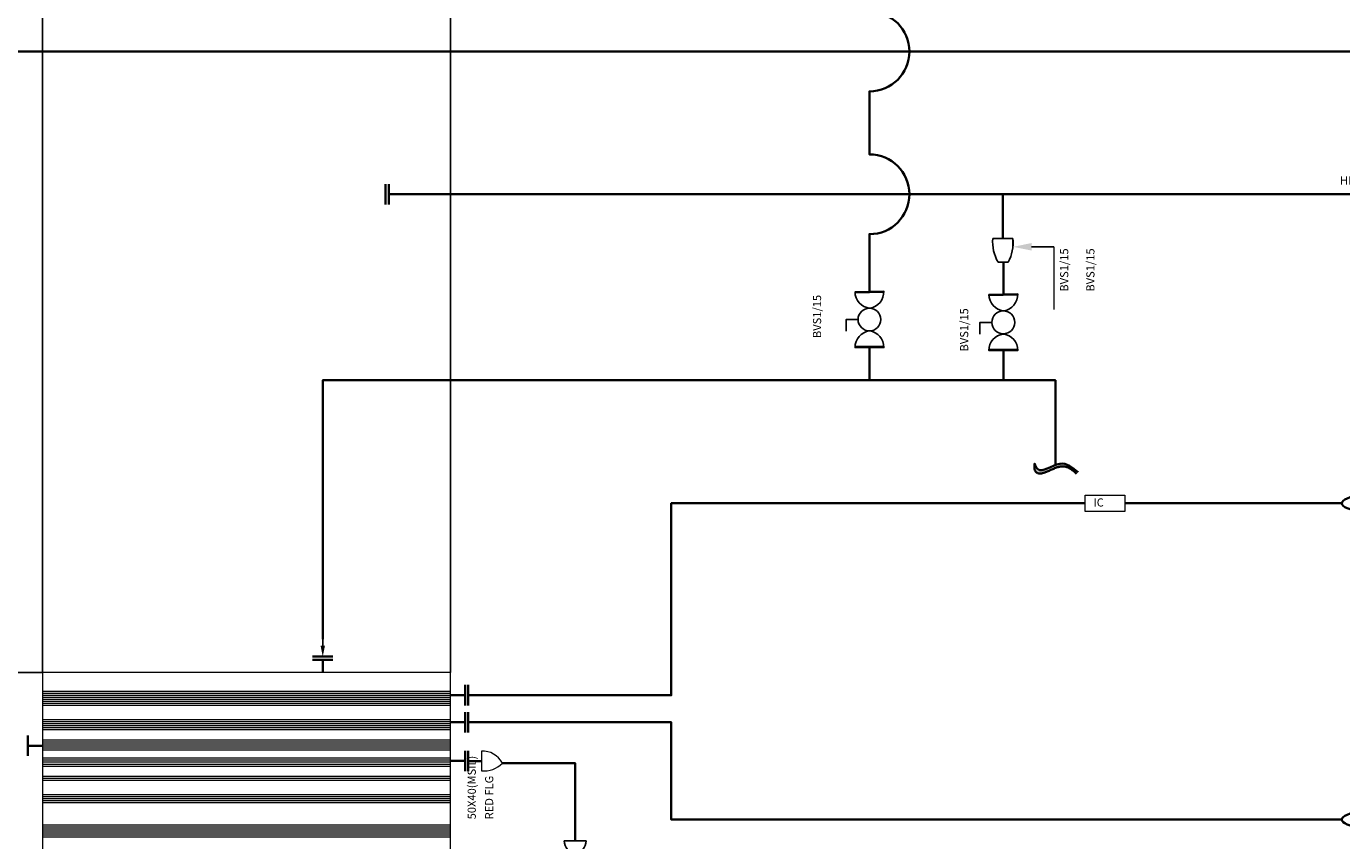
# Model space of a CAD drawing. Units: millimetres. Extents: x 353872 to 441597, y 126154 to 187356.
# Tile 24 of 28: x 399262 to 415084, y 165906 to 175703. Entities that reach past the tile are written whole.
import ezdxf

# ---------------------------------------------------------------- set-up
doc = ezdxf.new("R2010")
doc.units = ezdxf.units.MM
for name, color, linetype, lineweight in [('A-ANNO-DIMS', 2, 'Continuous', 18), ('P-ANNO-SYMB', 7, 'Continuous', 18), ('P-ANNO-TEXT', 7, 'Continuous', 25), ('P-INST-SIGN', 4, 'Continuous', 18), ('P-PIPE', 3, 'Continuous', 35), ('P-PIPE-FITT', 6, 'Continuous', 25), ('P-SYMB-PATT', 8, 'Continuous', 13), ('P-VALV', 2, 'Continuous', 25)]:
    doc.layers.add(name, color=color, linetype=linetype, lineweight=lineweight)
doc.layers.add('AC-UINT', color=2, linetype='Continuous')
doc.styles.get("Standard").update_dxf_attribs({"font": 'arial.ttf'})
doc.dimstyles.get("Standard").update_dxf_attribs({"dimtxt": 0.18, "dimasz": 0.18, "dimexe": 0.18, "dimexo": 0.0625, "dimgap": 0.09, "dimtad": 0, "dimtih": 1, "dimtoh": 1, "dimdec": 4, "dimzin": 0, "dimdsep": 46, "dimtxsty": 'Standard', "dimcen": 0.09, "dimadec": 0, "dimazin": 0, "dimtfac": 1, "dimtdec": 4, "dimtofl": 0, "dimtmove": 0, "dimatfit": 3, "dimfxl": 1, "dimtolj": 1, "dimtzin": 0, "dimarcsym": 0})

# ---------------------------------------------------------------- blocks, each defined once
blk = doc.blocks.new('DFSG')
at = {"layer": 'AC-UINT', "ltscale": 3}
blk.add_line((94.324, -27.16), (94.091, -27.16), dxfattribs=at)
blk.add_solid([(94.091, -27.121), (94.091, -27.199), (93.897, -27.16)], dxfattribs=at)
blk = doc.blocks.new('VALVE-B')
for points in [[(0, 12), (347, 12)], [(0, 8), (347, 8)], [(0, 4), (0, 0), (347, 0), (347, 5)], [(0, 4), (0, 4), (343, 4), (347, 4)]]:
    blk.add_lwpolyline(points)
for centre, radius, start, end in [((199, 2), 199, 97.3612, 180.5798), ((149, 3), 198, 359.2193, 82.8397)]:
    blk.add_arc(centre, radius, start, end)
blk = doc.blocks.new('VALVE-P')
blk.add_lwpolyline([(264, 173), (0, 173)])
for centre, radius, start, end in [((199, 188), 200, 184.2463, 250.3444), ((64, 189), 201, 289.8639, 355.5453)]:
    blk.add_arc(centre, radius, start, end)
blk = doc.blocks.new('*D33')
at = {"layer": 'A-ANNO-DIMS', "color": 0, "lineweight": -2, "transparency": 16777216}
for p, q in [((399457, 167930), (399457, 186546)), ((399457, 186546), (401910, 186546)), ((404363, 186546), (401911, 186546)), ((404363, 167930), (404363, 186546))]:
    blk.add_line(p, q, dxfattribs=at)
at = {"layer": 'A-ANNO-DIMS', "color": 0, "transparency": 16777216}
for points in [[(399457, 186546), (399457, 186546), (399457, 186546)], [(404363, 186546), (404363, 186546), (404363, 186546)]]:
    blk.add_solid(points, dxfattribs=at)
at = {"layer": 'Defpoints', "color": 0, "transparency": 16777216}
for p in [(404363, 186546), (399457, 167930), (404363, 167930)]:
    blk.add_point(p, dxfattribs=at)
at = {"layer": 'A-ANNO-DIMS', "color": 0, "transparency": 16777216, "insert": (401910, 186546), "char_height": 0.18, "attachment_point": 5}
blk.add_mtext('\\A1;4906', dxfattribs=at)
blk = doc.blocks.new('*D34')
at = {"layer": 'A-ANNO-DIMS', "color": 0, "lineweight": -2, "transparency": 16777216}
for p, q in [((399457, 167930), (356736, 167930)), ((356737, 167930), (356737, 163994)), ((356737, 160058), (356737, 163994)), ((399457, 160058), (356736, 160058))]:
    blk.add_line(p, q, dxfattribs=at)
at = {"layer": 'A-ANNO-DIMS', "color": 0, "transparency": 16777216}
for points in [[(356737, 167930), (356737, 167930), (356737, 167930)], [(356737, 160058), (356737, 160058), (356737, 160058)]]:
    blk.add_solid(points, dxfattribs=at)
at = {"layer": 'Defpoints', "color": 0, "transparency": 16777216}
for p in [(399457, 167930), (356737, 160058), (399457, 160058)]:
    blk.add_point(p, dxfattribs=at)
at = {"layer": 'A-ANNO-DIMS', "color": 0, "transparency": 16777216, "insert": (356737, 163994), "char_height": 0.18, "attachment_point": 5}
blk.add_mtext('\\A1;7872', dxfattribs=at)

msp = doc.modelspace()

# ---------------------------------------------------------------- hatches: boundary and pattern name
at = {"layer": 'P-SYMB-PATT'}
h = msp.add_hatch(color=256, dxfattribs=at)
h.dxf.hatch_style = 1
edge = h.paths.add_edge_path()
edge.add_spline(control_points=[(411390.89, 170443.52), (411390.67, 170440.97), (411390.44, 170438.39), (411389.76, 170430.59), (411389.33, 170425.32), (411388.62, 170414.26), (411388.36, 170408.48), (411388.27, 170396.91), (411388.44, 170391.13), (411389.36, 170382.04), (411389.81, 170378.82), (411390.94, 170373.15), (411391.51, 170370.72), (411392.96, 170365.81), (411393.81, 170363.36), (411396.48, 170356.98), (411398.56, 170353.08), (411403.61, 170345.73), (411406.6, 170342.29), (411413.25, 170336.23), (411416.92, 170333.63), (411424.5, 170329.4), (411428.41, 170327.76), (411436.16, 170325.33), (411440, 170324.52), (411447.5, 170323.5), (411451.17, 170323.28), (411461.46, 170323.25), (411467.9, 170323.94), (411480.65, 170326.14), (411486.96, 170327.66), (411499.68, 170331.29), (411506.08, 170333.4), (411519.07, 170338.07), (411525.65, 170340.62), (411546.51, 170349.09), (411561.13, 170355.56), (411590.78, 170368.69), (411605.81, 170375.36), (411635.44, 170387.63), (411650.05, 170393.24), (411670.51, 170399.85), (411676.94, 170401.73), (411687.59, 170404.43), (411691.93, 170405.39), (411699.54, 170406.83), (411702.88, 170407.37), (411709.47, 170408.22), (411712.7, 170408.53), (411722.23, 170409.19), (411728.37, 170409.22), (411744.84, 170408.35), (411754.86, 170406.72), (411774.52, 170401.58), (411784.16, 170398.07), (411803.36, 170389.36), (411812.91, 170384.17), (411832.06, 170372.4), (411841.65, 170365.83), (411864.69, 170349.03), (411878.19, 170338.36), (411893.02, 170320.82)], knot_values=[0, 0, 0, 0, 1.45657696, 1.45657696, 4.36973087, 4.36973087, 7.5343006, 7.5343006, 10.69887033, 10.69887033, 12.40671205, 12.40671205, 13.63901259, 13.63901259, 14.87131314, 14.87131314, 16.90061252, 16.90061252, 18.92991189, 18.92991189, 20.95921127, 20.95921127, 22.98851065, 22.98851065, 25.01781003, 25.01781003, 27.04710941, 27.04710941, 30.82532254, 30.82532254, 34.60353567, 34.60353567, 38.38174881, 38.38174881, 42.15996194, 42.15996194, 50.18983557, 50.18983557, 58.21970919, 58.21970919, 66.24958282, 66.24958282, 70.07411996, 70.07411996, 72.8401263, 72.8401263, 75.12034604, 75.12034604, 77.40056578, 77.40056578, 81.96100526, 81.96100526, 89.95516575, 89.95516575, 97.94932623, 97.94932623, 105.94348671, 105.94348671, 113.9376472, 113.9376472, 125.00201057, 125.00201057, 125.00201057, 125.00201057], degree=3, periodic=0)
edge.add_line((411893.02, 170320.82), (411913.35, 170339.3))
edge.add_spline(control_points=[(411913.35, 170339.3), (411845.38, 170395.98), (411763.83, 170463.97), (411657.92, 170432.84), (411640.09, 170426.25)], knot_values=[65.29657048, 65.29657048, 65.29657048, 65.29657048, 118.21354525, 128.78520648, 128.78520648, 128.78520648, 128.78520648], degree=3, periodic=0)
edge.add_spline(control_points=[(411640.09, 170426.25), (411557, 170395.56), (411440.95, 170314.41), (411400.77, 170418.04), (411390.89, 170443.52)], knot_values=[0, 0, 0, 0, 49.23816608, 65.29657048, 65.29657048, 65.29657048, 65.29657048], degree=3, periodic=0)

# ---------------------------------------------------------------- linework, layer by layer
at = {"layer": 'P-ANNO-SYMB'}
msp.add_line((411623.42, 173050.35), (411623.42, 172295.58), dxfattribs=at)
at = {"layer": 'P-INST-SIGN'}
for p, q in [((399457.15, 167706.61), (404363.17, 167706.61)), ((399457.15, 167682.23), (404363.17, 167682.23)), ((399457.15, 167657.84), (404363.17, 167657.84)), ((399457.15, 167633.45), (404363.17, 167633.45)), ((399457.15, 167633.45), (404363.17, 167633.45)), ((399457.15, 167609.06), (404363.17, 167609.06)), ((399457.15, 167584.67), (404363.17, 167584.67)), ((399457.15, 167560.28), (404363.17, 167560.28)), ((399457.15, 167560.28), (404363.17, 167560.28)), ((399457.15, 167535.9), (404363.17, 167535.9)), ((399457.15, 167365.18), (404363.17, 167365.18)), ((399457.15, 167340.79), (404363.17, 167340.79)), ((399457.15, 167316.4), (404363.17, 167316.4)), ((399457.15, 167292.01), (404363.17, 167292.01)), ((399457.15, 167267.62), (404363.17, 167267.62)), ((399457.15, 167243.23), (404363.17, 167243.23)), ((399457.15, 167121.29), (404363.17, 167121.29)), ((399457.15, 167096.9), (404363.17, 167096.9)), ((399457.15, 167072.52), (404363.17, 167072.52)), ((399457.15, 167048.13), (404363.17, 167048.13)), ((399457.15, 167023.74), (404363.17, 167023.74)), ((399457.15, 166999.35), (404363.17, 166999.35)), ((404736.17, 166983.02), (404736.17, 166745.9)), ((399457.15, 166901.8), (404363.17, 166901.8)), ((399457.15, 166877.41), (404363.17, 166877.41)), ((399457.15, 166853.02), (404363.17, 166853.02)), ((399457.15, 166828.63), (404363.17, 166828.63)), ((399457.15, 166804.24), (404363.17, 166804.24)), ((399457.15, 166682.3), (404363.17, 166682.3)), ((399457.15, 166657.91), (404363.17, 166657.91)), ((399457.15, 166657.91), (404363.17, 166657.91)), ((399457.15, 166633.52), (404363.17, 166633.52)), ((399457.15, 166462.8), (404363.17, 166462.8)), ((399457.15, 166438.42), (404363.17, 166438.42)), ((399457.15, 166414.03), (404363.17, 166414.03)), ((399457.15, 166389.64), (404363.17, 166389.64)), ((399457.15, 166365.25), (404363.17, 166365.25)), ((399457.15, 166096.98), (404363.17, 166096.98)), ((399457.15, 166072.59), (404363.17, 166072.59)), ((399457.15, 166048.2), (404363.17, 166048.2)), ((399457.15, 166048.2), (404363.17, 166048.2)), ((399457.15, 166023.81), (404363.17, 166023.81)), ((399457.15, 165999.42), (404363.17, 165999.42)), ((399457.15, 165975.04), (404363.17, 165975.04)), ((399457.15, 165950.65), (404363.17, 165950.65))]:
    msp.add_line(p, q, dxfattribs=at)
for points in [[(411999.14, 170063.27), (412475.78, 170063.27), (412475.78, 169866.13), (411999.14, 169866.13)], [(404363.17, 167929.97), (399457.15, 167929.97), (399457.15, 160058.19), (404363.17, 160058.19)]]:
    msp.add_lwpolyline(points, close=True, dxfattribs=at)
for centre, radius, start, end in [((404752.45, 166718.18), 265.34, 27.376995, 93.518711), ((404764.38, 167054.18), 309.56, 264.770963, 316.27178)]:
    msp.add_arc(centre, radius, start, end, dxfattribs=at)
at = {"layer": 'P-PIPE'}
for p, q in [((403583.29, 173805.12), (403583.29, 173560.36)), ((403622.45, 173805.12), (403622.45, 173560.36)), ((426420.76, 173682.74), (403622.45, 173682.74)), ((411008.36, 173150.27), (411008.36, 173682.74)), ((411014.55, 172476.18), (411014.55, 172864.89)), ((409404.23, 171839.16), (409404.23, 171444.56)), ((411014.53, 171789.73), (411014.53, 171444.56)), ((415084.48, 169964.7), (412475.78, 169964.7)), ((402950.3, 168120.52), (402705.54, 168120.52)), ((402950.3, 168081.36), (402705.54, 168081.36)), ((402827.92, 168081.36), (402827.92, 167929.97)), ((404538.96, 167779.19), (404538.96, 167534.43)), ((404578.12, 167779.19), (404578.12, 167534.43)), ((404363.17, 167657.84), (404538.96, 167657.84)), ((404538.96, 167452.85), (404538.96, 167208.09)), ((404578.12, 167452.85), (404578.12, 167208.09)), ((404363.17, 167331.49), (404538.96, 167331.49)), ((399281.36, 166926.77), (399281.36, 167171.53)), ((399457.15, 167048.13), (399281.36, 167048.13)), ((404538.96, 166986.76), (404538.96, 166742)), ((404578.12, 166986.76), (404578.12, 166742)), ((404363.17, 166865.41), (404538.96, 166865.41)), ((404578.12, 166864.38), (404736.17, 166864.38))]:
    msp.add_line(p, q, dxfattribs=at)
msp.add_lwpolyline([(426420.76, 177114.41), (409404.23, 177114.41), (409404.23, 175879.94, -1), (409404.23, 174919.83), (409404.23, 174162.79, -1), (409404.23, 173202.69), (409404.23, 172914.66), (409404.23, 172512.05)], format="xyb", dxfattribs=at)
for points in [[(393066.71, 149319.73), (393066.71, 175399.89), (426420.76, 175399.89)], [(402828.13, 168331.12), (402827.92, 171444.56), (411640.09, 171444.56), (411640.09, 170426.25)], [(411999.14, 169964.7), (407132.63, 169964.7), (407019.22, 169964.7), (407019.22, 167656.81), (405749.06, 167656.81), (404578.12, 167656.81)], [(415084.48, 166160.17), (411014.25, 166160.17), (407019.22, 166160.17), (407019.22, 167330.47), (404578.12, 167330.47)], [(404988.08, 166840.2), (405863.95, 166840.2), (405863.95, 165906.19)]]:
    msp.add_lwpolyline(points, dxfattribs=at)
for centre in [(415913.9, 169964.7), (415913.9, 169964.7), (415913.9, 166160.17), (415913.9, 166160.17)]:
    msp.add_ellipse(centre, major_axis=(829.42, 0), ratio=0.18269243, dxfattribs=at)
msp.add_open_spline([(411913.35, 170339.3), (411845.38, 170395.98), (411700.58, 170516.7), (411447.45, 170297.63), (411400.77, 170418.04), (411390.89, 170443.52), (411390.67, 170440.97), (411390.44, 170438.39), (411389.76, 170430.59), (411389.33, 170425.32), (411388.62, 170414.26), (411388.36, 170408.48), (411388.27, 170396.91), (411388.44, 170391.13), (411389.36, 170382.04), (411389.81, 170378.82), (411390.94, 170373.15), (411391.51, 170370.72), (411392.96, 170365.81), (411393.81, 170363.36), (411396.48, 170356.98), (411398.56, 170353.08), (411403.61, 170345.73), (411406.6, 170342.29), (411413.25, 170336.23), (411416.92, 170333.63), (411424.5, 170329.4), (411428.41, 170327.76), (411436.16, 170325.33), (411440, 170324.52), (411447.5, 170323.5), (411451.17, 170323.28), (411461.46, 170323.25), (411467.9, 170323.94), (411480.65, 170326.14), (411486.96, 170327.66), (411499.68, 170331.29), (411506.08, 170333.4), (411519.07, 170338.07), (411525.65, 170340.62), (411546.51, 170349.09), (411561.13, 170355.56), (411590.78, 170368.69), (411605.81, 170375.36), (411635.44, 170387.63), (411650.05, 170393.24), (411670.51, 170399.85), (411676.94, 170401.73), (411687.59, 170404.43), (411691.93, 170405.39), (411699.54, 170406.83), (411702.88, 170407.37), (411709.47, 170408.22), (411712.7, 170408.53), (411722.23, 170409.19), (411728.37, 170409.22), (411744.84, 170408.35), (411754.86, 170406.72), (411774.52, 170401.58), (411784.16, 170398.07), (411803.36, 170389.36), (411812.91, 170384.17), (411832.06, 170372.4), (411841.65, 170365.83), (411864.69, 170349.03), (411878.19, 170338.36), (411893.02, 170320.82)], degree=3, knots=[0, 0, 0, 0, 346.87515529, 738.93353045, 844.19770217, 844.19770217, 844.19770217, 845.65427913, 845.65427913, 848.56743304, 848.56743304, 851.73200277, 851.73200277, 854.8965725, 854.8965725, 856.60441422, 856.60441422, 857.83671477, 857.83671477, 859.06901531, 859.06901531, 861.09831469, 861.09831469, 863.12761407, 863.12761407, 865.15691345, 865.15691345, 867.18621283, 867.18621283, 869.2155122, 869.2155122, 871.24481158, 871.24481158, 875.02302472, 875.02302472, 878.80123785, 878.80123785, 882.57945098, 882.57945098, 886.35766411, 886.35766411, 894.38753774, 894.38753774, 902.41741137, 902.41741137, 910.44728499, 910.44728499, 914.27182214, 914.27182214, 917.03782847, 917.03782847, 919.31804821, 919.31804821, 921.59826795, 921.59826795, 926.15870744, 926.15870744, 934.15286792, 934.15286792, 942.1470284, 942.1470284, 950.14118889, 950.14118889, 958.13534937, 958.13534937, 969.19971274, 969.19971274, 969.19971274, 969.19971274], dxfattribs=at)
at = {"layer": 'P-VALV'}
for p, q in [((411130.35, 173150.27), (410886.38, 173150.27)), ((411130.35, 173058.5), (411130.35, 173151.98))]:
    msp.add_line(p, q, dxfattribs=at)
for points in [[(410950.47, 172864.89), (411014.55, 172864.89), (411072.45, 172864.89)], [(409266.91, 172175.6), (409123.61, 172175.6), (409123.61, 172034.91)], [(410876.15, 172141), (410731.72, 172141), (410731.72, 171999.19)]]:
    msp.add_lwpolyline(points, dxfattribs=at)
for centre, radius in [((409403.76, 172175.6), 136.85), ((411014.08, 172141), 137.93)]:
    msp.add_circle(centre, radius, dxfattribs=at)
for centre, radius, start, end in [((411379.15, 173111.03), 494.32, 175.447638, 209.864188), ((410628.49, 173103.52), 504.03, 331.741199, 5.321321)]:
    msp.add_arc(centre, radius, start, end, dxfattribs=at)

# ---------------------------------------------------------------- block references
at = {"layer": 'P-PIPE-FITT', "xscale": 1154.295526641529, "yscale": 1154.295526641529, "zscale": 1154.295526641529}
msp.add_blockref('DFSG', (302746.01, 204401.14), dxfattribs=at)
at = {"layer": 'P-PIPE-FITT', "xscale": 677.5688707767378, "yscale": 677.5688707767378, "zscale": 677.5688707767378, "rotation": 90.000000000006}
msp.add_blockref('DFSG', (384425.28, 104499.16), dxfattribs=at)
at = {"layer": 'P-VALV'}
for p, rotation in [((409577.1, 172515.99), 181.3019170021721), ((411187.42, 172483.84), 181.301917002174)]:
    msp.add_blockref('VALVE-B', p, dxfattribs=dict(at, rotation=rotation))
for name, p in [('VALVE-B', (409230.59, 171839.16)), ('VALVE-B', (410840.92, 171802.1)), ('VALVE-P', (405732.05, 165733.02))]:
    msp.add_blockref(name, p, dxfattribs=at)

# ---------------------------------------------------------------- texts
at = {"layer": 'P-ANNO-TEXT'}
for s, p in [('HDPE/100', (415064.35, 173799.23)), ('IC', (412098.35, 169925.94))]:
    msp.add_text(s, height=98.09, dxfattribs=at).set_placement(p)
for s, height, p in [('BVS1/15', 98.09, (411795.78, 172511.53)), ('BVS1/15', 98.09, (412110.58, 172511.53)), ('BVS1/15', 98.09, (408822.67, 171952.34)), ('BVS1/15', 98.09, (410592.55, 171791.58)), ('50X40(MSIL)', 98.0901, (404668.96, 166163.36)), ('RED FLG', 98.09, (404878.87, 166163.36))]:
    msp.add_text(s, height=height, rotation=90, dxfattribs=at).set_placement(p)

# ---------------------------------------------------------------- dimensions: what is measured, and where the dimension line sits
at = {"layer": 'A-ANNO-DIMS'}
dim = msp.add_linear_dim(base=(404363.17, 186546.05), p1=(399457.15, 167929.97), p2=(404363.17, 167929.97), dimstyle='Standard', override={"dimdec": 0, "dimlfac": 1, "dimrnd": 0, "dimzin": 0, "dimdsep": 46, "dimlunit": 2}, dxfattribs=at)
dim.commit()
dim.dimension.update_dxf_attribs({"geometry": '*D33', "text_midpoint": (401910.16, 186546.05)})
dim = msp.add_linear_dim(base=(356736.55, 160058.19), p1=(399457.15, 167929.97), p2=(399457.15, 160058.19), angle=90, dimstyle='Standard', override={"dimdec": 0, "dimlfac": 1, "dimrnd": 0, "dimzin": 0, "dimdsep": 46, "dimlunit": 2}, dxfattribs=at)
dim.commit()
dim.dimension.update_dxf_attribs({"geometry": '*D34', "text_midpoint": (356736.55, 163994.08)})

doc.saveas('drawing.dxf')
